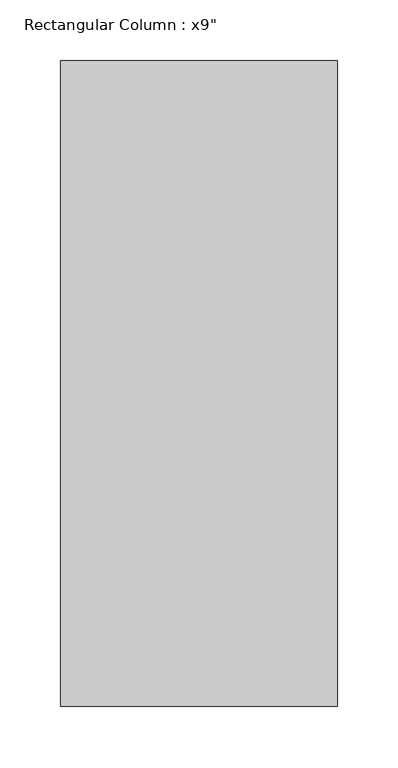
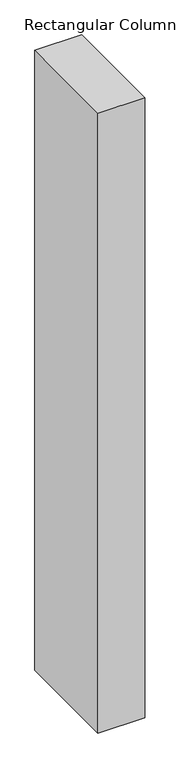
"""IFC4 building model written with IfcOpenShell, lengths in millimetres: column geometry."""

from ifc_helpers import new_model, si_unit, frame, origin, place, context, project, spatial, polyline, outline, extrude, source, transform, mapped, element, save


def column_b42c64cd(model_context):
    return source(origin(), model_context, "Body", "SweptSolid", [
        extrude(outline(polyline([(114.3, 266.7), (114.3, -266.7), (-114.3, -266.7), (-114.3, 266.7), (114.3, 266.7)])), frame((0.0, 0.0, 3200.4), z_axis=(0.0, 0.0, 1.0), x_axis=(1.0, 0.0, 0.0)), (0.0, 0.0, 1.0), 3200.4),
    ])


if __name__ == "__main__":
    model = new_model("IFC4")
    model_context = context("Model", 3, world=origin())
    ifc_project = project(units=[si_unit("LENGTHUNIT", "METRE", prefix="MILLI")], contexts=[model_context])
    site = spatial("IfcSite", under=ifc_project)
    building = spatial("IfcBuilding", under=site)
    placement = place(None, origin())
    column_shape = column_b42c64cd(model_context)
    element("IfcColumn", 1, ObjectType="Rectangular Column : x9\"", at=placement, inside=building, context=model_context, shape_type="MappedRepresentation", body=[
        mapped(column_shape, transform((0.0, 0.0, 0.0), x_axis=(1.0, 0.0, 0.0), y_axis=(0.0, 1.0, 0.0), z_axis=(0.0, 0.0, 1.0))),
    ])
    save(model, "model.ifc")

# Revit data of these elements
# Type "Rectangular Column : x9\""
#   Assembly Code = "B1010200"
#   Depth = 1' - 9"
#   Offset Base = 0' - 0"
#   Offset Top = 0' - 0"
#   Width = 0' - 9"
#   Material = none
